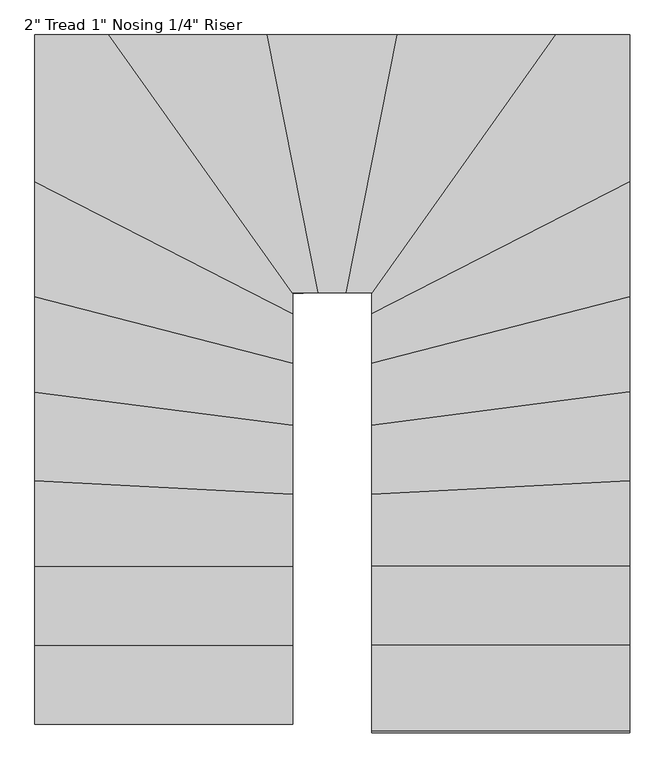
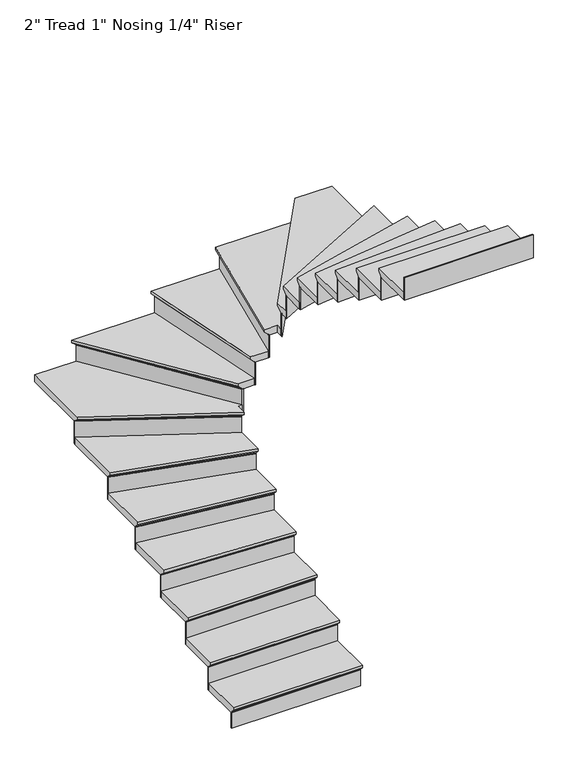
"""IFC4 building model written with IfcOpenShell, lengths in millimetres: stair flight geometry."""

from ifc_helpers import new_model, si_unit, origin, place, context, project, spatial, faceted_brep, source, transform, mapped, element, save


def stair_flight_079dc026(model_context):
    return source(origin(), model_context, "Body", "Brep", [
        faceted_brep([(-8021.860887, -4607.8089531, 150.2833333), (-8021.860887, -4607.8089531, 169.3333333), (-8936.260887, -4607.8089531, 169.3333333), (-8936.260887, -4607.8089531, 150.2833333), (-8021.860887, -4582.4089531, 124.8833333), (-8936.260887, -4582.4089531, 124.8833333), (-8021.860887, -4303.0089531, 169.3333333), (-8936.260887, -4303.0089531, 169.3333333), (-8936.260887, -4582.4089531, 118.5333333), (-8936.260887, -4303.0089531, 118.5333333), (-8021.860887, -4303.0089531, 118.5333333), (-8021.860887, -4582.4089531, 118.5333333)], [[[0, 1, 2, 3]], [[4, 0, 3, 5]], [[2, 1, 6, 7]], [[8, 9, 10, 11]], [[2, 7, 9, 8, 5, 3]], [[8, 11, 4, 5]], [[6, 1, 0, 4, 11, 10]], [[7, 6, 10, 9]]]),
        faceted_brep([(-8021.860887, -4582.4089531, 118.5333333), (-8021.860887, -4582.4089531, 0.0), (-8021.860887, -4576.0589531, 0.0), (-8021.860887, -4576.0589531, 118.5333333), (-8936.260887, -4582.4089531, 118.5333333), (-8936.260887, -4576.0589531, 118.5333333), (-8936.260887, -4576.0589531, 0.0), (-8936.260887, -4582.4089531, 0.0)], [[[0, 1, 2, 3]], [[4, 5, 6, 7]], [[1, 0, 4, 7]], [[2, 1, 7, 6]], [[3, 2, 6, 5]], [[0, 3, 5, 4]]]),
        faceted_brep([(-8021.860887, -4303.0089531, 287.8666667), (-8021.860887, -4303.0089531, 118.5333333), (-8021.860887, -4296.6589531, 118.5333333), (-8021.860887, -4296.6589531, 287.8666667), (-8936.260887, -4303.0089531, 287.8666667), (-8936.260887, -4296.6589531, 287.8666667), (-8936.260887, -4296.6589531, 118.5333333), (-8936.260887, -4303.0089531, 118.5333333)], [[[0, 1, 2, 3]], [[4, 5, 6, 7]], [[1, 0, 4, 7]], [[2, 1, 7, 6]], [[3, 2, 6, 5]], [[0, 3, 5, 4]]]),
        faceted_brep([(-8936.260887, -4328.4089531, 338.6666667), (-8021.860887, -4328.4089531, 338.6666667), (-8021.860887, -4023.6089531, 338.6666667), (-8936.260887, -4023.6089531, 338.6666667), (-8936.260887, -4303.0089531, 287.8666667), (-8936.260887, -4023.6089531, 287.8666667), (-8021.860887, -4023.6089531, 287.8666667), (-8021.860887, -4303.0089531, 287.8666667), (-8936.260887, -4303.0089531, 294.2166667), (-8936.260887, -4328.4089531, 319.6166667), (-8021.860887, -4303.0089531, 294.2166667), (-8021.860887, -4328.4089531, 319.6166667)], [[[0, 1, 2, 3]], [[4, 5, 6, 7]], [[0, 3, 5, 4, 8, 9]], [[4, 7, 10, 8]], [[2, 1, 11, 10, 7, 6]], [[3, 2, 6, 5]], [[11, 1, 0, 9]], [[10, 11, 9, 8]]]),
        faceted_brep([(-8021.860887, -4023.6089531, 457.2), (-8021.860887, -4023.6089531, 287.8666667), (-8021.860887, -4017.2589531, 287.8666667), (-8021.860887, -4017.2589531, 457.2), (-8936.260887, -4023.6089531, 457.2), (-8936.260887, -4017.2589531, 457.2), (-8936.260887, -4017.2589531, 287.8666667), (-8936.260887, -4023.6089531, 287.8666667)], [[[0, 1, 2, 3]], [[4, 5, 6, 7]], [[1, 0, 4, 7]], [[2, 1, 7, 6]], [[3, 2, 6, 5]], [[0, 3, 5, 4]]]),
        faceted_brep([(-8936.260887, -4049.0089531, 508.0), (-8021.860887, -4049.0089531, 508.0), (-8021.860887, -3767.9417916, 508.0), (-8936.260887, -3720.4075212, 508.0), (-8936.260887, -4023.6089531, 457.2), (-8936.260887, -3720.4075212, 457.2), (-8021.860887, -3767.9417916, 457.2), (-8021.860887, -4023.6089531, 457.2), (-8936.260887, -4023.6089531, 463.55), (-8936.260887, -4049.0089531, 488.95), (-8021.860887, -4023.6089531, 463.55), (-8021.860887, -4049.0089531, 488.95)], [[[0, 1, 2, 3]], [[4, 5, 6, 7]], [[0, 3, 5, 4, 8, 9]], [[4, 7, 10, 8]], [[2, 1, 11, 10, 7, 6]], [[3, 2, 6, 5]], [[11, 1, 0, 9]], [[10, 11, 9, 8]]]),
        faceted_brep([(-8021.860887, -3767.9417916, 626.5333333), (-8021.860887, -3767.9417916, 457.2), (-8021.860887, -3761.5832175, 457.2), (-8021.860887, -3761.5832175, 626.5333333), (-8936.260887, -3720.4075212, 626.5333333), (-8936.260887, -3714.0489471, 626.5333333), (-8936.260887, -3714.0489471, 457.2), (-8936.260887, -3720.4075212, 457.2)], [[[0, 1, 2, 3]], [[4, 5, 6, 7]], [[1, 0, 4, 7]], [[2, 1, 7, 6]], [[3, 2, 6, 5]], [[0, 3, 5, 4]]]),
        faceted_brep([(-8936.260887, -3745.8418179, 677.3333333), (-8021.860887, -3793.3760883, 677.3333333), (-8021.860887, -3523.7750918, 677.3333333), (-8936.260887, -3405.4190402, 677.3333333), (-8936.260887, -3720.4075212, 626.5333333), (-8936.260887, -3405.4190402, 626.5333333), (-8021.860887, -3523.7750918, 626.5333333), (-8021.860887, -3767.9417916, 626.5333333), (-8936.260887, -3720.4075212, 632.8833333), (-8936.260887, -3745.8418179, 658.2833333), (-8021.860887, -3767.9417916, 632.8833333), (-8021.860887, -3793.3760883, 658.2833333)], [[[0, 1, 2, 3]], [[4, 5, 6, 7]], [[0, 3, 5, 4, 8, 9]], [[4, 7, 10, 8]], [[2, 1, 11, 10, 7, 6]], [[3, 2, 6, 5]], [[11, 1, 0, 9]], [[10, 11, 9, 8]]]),
        faceted_brep([(-8021.860887, -3523.7750918, 795.8666667), (-8021.860887, -3523.7750918, 626.5333333), (-8021.860887, -3517.37212, 626.5333333), (-8021.860887, -3517.37212, 795.8666667), (-8936.260887, -3405.4190402, 795.8666667), (-8936.260887, -3399.0160684, 795.8666667), (-8936.260887, -3399.0160684, 626.5333333), (-8936.260887, -3405.4190402, 626.5333333)], [[[0, 1, 2, 3]], [[4, 5, 6, 7]], [[1, 0, 4, 7]], [[2, 1, 7, 6]], [[3, 2, 6, 5]], [[0, 3, 5, 4]]]),
        faceted_brep([(-8936.260887, -3431.0309273, 846.6666667), (-8021.860887, -3549.3869789, 846.6666667), (-8021.860887, -3302.1478693, 846.6666667), (-8936.260887, -3067.0174219, 846.6666667), (-8936.260887, -3405.4190402, 795.8666667), (-8936.260887, -3067.0174219, 795.8666667), (-8021.860887, -3302.1478693, 795.8666667), (-8021.860887, -3523.7750918, 795.8666667), (-8936.260887, -3405.4190402, 802.2166667), (-8936.260887, -3431.0309273, 827.6166667), (-8021.860887, -3523.7750918, 802.2166667), (-8021.860887, -3549.3869789, 827.6166667)], [[[0, 1, 2, 3]], [[4, 5, 6, 7]], [[0, 3, 5, 4, 8, 9]], [[4, 7, 10, 8]], [[2, 1, 11, 10, 7, 6]], [[3, 2, 6, 5]], [[11, 1, 0, 9]], [[10, 11, 9, 8]]]),
        faceted_brep([(-8021.860887, -3302.1478693, 965.2), (-8021.860887, -3302.1478693, 795.8666667), (-8021.860887, -3295.5912925, 795.8666667), (-8021.860887, -3295.5912925, 965.2), (-8936.260887, -3067.0174219, 965.2), (-8936.260887, -3060.4608451, 965.2), (-8936.260887, -3060.4608451, 795.8666667), (-8936.260887, -3067.0174219, 795.8666667)], [[[0, 1, 2, 3]], [[4, 5, 6, 7]], [[1, 0, 4, 7]], [[2, 1, 7, 6]], [[3, 2, 6, 5]], [[0, 3, 5, 4]]]),
        faceted_brep([(-8936.260887, -3093.2437294, 1016.0), (-8021.860887, -3328.3741768, 1016.0), (-8021.860887, -3125.8012333, 1016.0), (-8936.260887, -2656.9766119, 1016.0), (-8936.260887, -3067.0174219, 965.2), (-8936.260887, -2656.9766119, 965.2), (-8021.860887, -3125.8012333, 965.2), (-8021.860887, -3302.1478693, 965.2), (-8936.260887, -3067.0174219, 971.55), (-8936.260887, -3093.2437294, 996.95), (-8021.860887, -3302.1478693, 971.55), (-8021.860887, -3328.3741768, 996.95)], [[[0, 1, 2, 3]], [[4, 5, 6, 7]], [[0, 3, 5, 4, 8, 9]], [[4, 7, 10, 8]], [[2, 1, 11, 10, 7, 6]], [[3, 2, 6, 5]], [[11, 1, 0, 9]], [[10, 11, 9, 8]]]),
        faceted_brep([(-8021.860887, -3125.8012333, 1134.5333333), (-8021.860887, -3125.8012333, 965.2), (-8021.860887, -3118.6652501, 965.2), (-8021.860887, -3118.6652501, 1134.5333333), (-8936.260887, -2656.9766119, 1134.5333333), (-8936.260887, -2649.8406288, 1134.5333333), (-8936.260887, -2649.8406288, 965.2), (-8936.260887, -2656.9766119, 965.2)], [[[0, 1, 2, 3]], [[4, 5, 6, 7]], [[1, 0, 4, 7]], [[2, 1, 7, 6]], [[3, 2, 6, 5]], [[0, 3, 5, 4]]]),
        faceted_brep([(-8642.5797533, -2165.6772612, 1185.3333333), (-8936.260887, -2165.6772612, 1185.3333333), (-8936.260887, -2685.5205445, 1185.3333333), (-8021.860887, -3154.3451658, 1185.3333333), (-8021.860887, -3080.0772612, 1185.3333333), (-7992.3058042, -3080.0772612, 1185.3333333), (-8936.260887, -2165.6772612, 1134.5333333), (-8642.5797533, -2165.6772612, 1134.5333333), (-7992.3058042, -3080.0772612, 1134.5333333), (-8021.860887, -3080.0772612, 1134.5333333), (-8021.860887, -3125.8012333, 1134.5333333), (-8936.260887, -2656.9766119, 1134.5333333), (-8936.260887, -2656.9766119, 1140.8833333), (-8936.260887, -2685.5205445, 1166.2833333), (-8021.860887, -3125.8012333, 1140.8833333), (-8021.860887, -3154.3451658, 1166.2833333)], [[[0, 1, 2, 3, 4, 5]], [[6, 7, 8, 9, 10, 11]], [[1, 0, 7, 6]], [[2, 1, 6, 11, 12, 13]], [[11, 10, 14, 12]], [[4, 3, 15, 14, 10, 9]], [[5, 4, 9, 8]], [[0, 5, 8, 7]], [[15, 3, 2, 13]], [[14, 15, 13, 12]]]),
        faceted_brep([(-7992.3058042, -3080.0772612, 1303.8666667), (-7992.3058042, -3080.0772612, 1134.5333333), (-7984.5138294, -3080.0772612, 1134.5333333), (-7984.5138294, -3080.0772612, 1303.8666667), (-8642.5797533, -2165.6772612, 1303.8666667), (-8634.7877785, -2165.6772612, 1303.8666667), (-8634.7877785, -2165.6772612, 1134.5333333), (-8642.5797533, -2165.6772612, 1134.5333333)], [[[0, 1, 2, 3]], [[4, 5, 6, 7]], [[1, 0, 4, 7]], [[2, 1, 7, 6]], [[3, 2, 6, 5]], [[0, 3, 5, 4]]]),
        faceted_brep([(-8673.7476525, -2165.6772612, 1354.6666667), (-8023.4737034, -3080.0772612, 1354.6666667), (-7905.8517171, -3080.0772612, 1354.6666667), (-8086.0925734, -2165.6772612, 1354.6666667), (-8642.5797533, -2165.6772612, 1303.8666667), (-8086.0925734, -2165.6772612, 1303.8666667), (-7905.8517171, -3080.0772612, 1303.8666667), (-7992.3058042, -3080.0772612, 1303.8666667), (-8642.5797533, -2165.6772612, 1310.2166667), (-8673.7476525, -2165.6772612, 1335.6166667), (-7992.3058042, -3080.0772612, 1310.2166667), (-8023.4737034, -3080.0772612, 1335.6166667)], [[[0, 1, 2, 3]], [[4, 5, 6, 7]], [[0, 3, 5, 4, 8, 9]], [[4, 7, 10, 8]], [[2, 1, 11, 10, 7, 6]], [[3, 2, 6, 5]], [[11, 1, 0, 9]], [[10, 11, 9, 8]]]),
        faceted_brep([(-7905.8517171, -3080.0772612, 1473.2), (-7905.8517171, -3080.0772612, 1303.8666667), (-7899.3795317, -3080.0772612, 1303.8666667), (-7899.3795317, -3080.0772612, 1473.2), (-8086.0925734, -2165.6772612, 1473.2), (-8079.620388, -2165.6772612, 1473.2), (-8079.620388, -2165.6772612, 1303.8666667), (-8086.0925734, -2165.6772612, 1303.8666667)], [[[0, 1, 2, 3]], [[4, 5, 6, 7]], [[1, 0, 4, 7]], [[2, 1, 7, 6]], [[3, 2, 6, 5]], [[0, 3, 5, 4]]]),
        faceted_brep([(-8111.9813152, -2165.6772612, 1524.0), (-7931.7404589, -3080.0772612, 1524.0), (-7806.6925734, -3080.0772612, 1524.0), (-7626.4517171, -2165.6772612, 1524.0), (-8086.0925734, -2165.6772612, 1473.2), (-7626.4517171, -2165.6772612, 1473.2), (-7806.6925734, -3080.0772612, 1473.2), (-7905.8517171, -3080.0772612, 1473.2), (-8086.0925734, -2165.6772612, 1479.55), (-8111.9813152, -2165.6772612, 1504.95), (-7905.8517171, -3080.0772612, 1479.55), (-7931.7404589, -3080.0772612, 1504.95)], [[[0, 1, 2, 3]], [[4, 5, 6, 7]], [[0, 3, 5, 4, 8, 9]], [[4, 7, 10, 8]], [[2, 1, 11, 10, 7, 6]], [[3, 2, 6, 5]], [[11, 1, 0, 9]], [[10, 11, 9, 8]]]),
        faceted_brep([(-7806.6925734, -3080.0772612, 1642.5333333), (-7806.6925734, -3080.0772612, 1473.2), (-7800.220388, -3080.0772612, 1473.2), (-7800.220388, -3080.0772612, 1642.5333333), (-7626.4517171, -2165.6772612, 1642.5333333), (-7619.9795317, -2165.6772612, 1642.5333333), (-7619.9795317, -2165.6772612, 1473.2), (-7626.4517171, -2165.6772612, 1473.2)], [[[0, 1, 2, 3]], [[4, 5, 6, 7]], [[1, 0, 4, 7]], [[2, 1, 7, 6]], [[3, 2, 6, 5]], [[0, 3, 5, 4]]]),
        faceted_brep([(-7652.3404589, -2165.6772612, 1693.3333333), (-7832.5813152, -3080.0772612, 1693.3333333), (-7742.460887, -3080.0772612, 1693.3333333), (-7742.460887, -3126.1727358, 1693.3333333), (-7059.4062224, -2165.6772612, 1693.3333333), (-7626.4517171, -2165.6772612, 1642.5333333), (-7059.4062224, -2165.6772612, 1642.5333333), (-7742.460887, -3126.1727358, 1642.5333333), (-7742.460887, -3080.0772612, 1642.5333333), (-7806.6925734, -3080.0772612, 1642.5333333), (-7626.4517171, -2165.6772612, 1648.8833333), (-7652.3404589, -2165.6772612, 1674.2833333), (-7806.6925734, -3080.0772612, 1648.8833333), (-7832.5813152, -3080.0772612, 1674.2833333)], [[[0, 1, 2, 3, 4]], [[5, 6, 7, 8, 9]], [[0, 4, 6, 5, 10, 11]], [[5, 9, 12, 10]], [[2, 1, 13, 12, 9, 8]], [[3, 2, 8, 7]], [[4, 3, 7, 6]], [[13, 1, 0, 11]], [[12, 13, 11, 10]]]),
        faceted_brep([(-7742.460887, -3126.1727358, 1811.8666667), (-7742.460887, -3126.1727358, 1642.5333333), (-7742.460887, -3137.1296282, 1642.5333333), (-7742.460887, -3137.1296282, 1811.8666667), (-7059.4062224, -2165.6772612, 1811.8666667), (-7051.6142476, -2165.6772612, 1811.8666667), (-7051.6142476, -2165.6772612, 1642.5333333), (-7059.4062224, -2165.6772612, 1642.5333333)], [[[0, 1, 2, 3]], [[4, 5, 6, 7]], [[1, 0, 4, 7]], [[2, 1, 7, 6]], [[3, 2, 6, 5]], [[0, 3, 5, 4]]]),
        faceted_brep([(-6828.060887, -2714.064477, 1862.6666667), (-6828.060887, -2165.6772612, 1862.6666667), (-7090.5741215, -2165.6772612, 1862.6666667), (-7742.460887, -3082.3451658, 1862.6666667), (-7742.460887, -3182.8890983, 1862.6666667), (-6828.060887, -2165.6772612, 1811.8666667), (-6828.060887, -2714.064477, 1811.8666667), (-7742.460887, -3182.8890983, 1811.8666667), (-7742.460887, -3126.1727358, 1811.8666667), (-7059.4062224, -2165.6772612, 1811.8666667), (-7059.4062224, -2165.6772612, 1818.2166667), (-7090.5741215, -2165.6772612, 1843.6166667), (-7742.460887, -3126.1727358, 1818.2166667), (-7742.460887, -3082.3451658, 1843.6166667)], [[[0, 1, 2, 3, 4]], [[5, 6, 7, 8, 9]], [[1, 0, 6, 5]], [[2, 1, 5, 9, 10, 11]], [[9, 8, 12, 10]], [[4, 3, 13, 12, 8, 7]], [[0, 4, 7, 6]], [[13, 3, 2, 11]], [[12, 13, 11, 10]]]),
        faceted_brep([(-7742.460887, -3182.8890983, 1981.2), (-7742.460887, -3182.8890983, 1811.8666667), (-7742.460887, -3190.0250815, 1811.8666667), (-7742.460887, -3190.0250815, 1981.2), (-6828.060887, -2714.064477, 1981.2), (-6828.060887, -2721.2004601, 1981.2), (-6828.060887, -2721.2004601, 1811.8666667), (-6828.060887, -2714.064477, 1811.8666667)], [[[0, 1, 2, 3]], [[4, 5, 6, 7]], [[1, 0, 4, 7]], [[2, 1, 7, 6]], [[3, 2, 6, 5]], [[0, 3, 5, 4]]]),
        faceted_brep([(-6828.060887, -2685.5205445, 2032.0), (-7742.460887, -3154.3451658, 2032.0), (-7742.460887, -3354.6004843, 2032.0), (-6828.060887, -3119.4700369, 2032.0), (-6828.060887, -2714.064477, 1981.2), (-6828.060887, -3119.4700369, 1981.2), (-7742.460887, -3354.6004843, 1981.2), (-7742.460887, -3182.8890983, 1981.2), (-6828.060887, -2714.064477, 1987.55), (-6828.060887, -2685.5205445, 2012.95), (-7742.460887, -3182.8890983, 1987.55), (-7742.460887, -3154.3451658, 2012.95)], [[[0, 1, 2, 3]], [[4, 5, 6, 7]], [[0, 3, 5, 4, 8, 9]], [[4, 7, 10, 8]], [[2, 1, 11, 10, 7, 6]], [[3, 2, 6, 5]], [[11, 1, 0, 9]], [[10, 11, 9, 8]]]),
        faceted_brep([(-7742.460887, -3354.6004843, 2150.5333333), (-7742.460887, -3354.6004843, 1981.2), (-7742.460887, -3361.1570611, 1981.2), (-7742.460887, -3361.1570611, 2150.5333333), (-6828.060887, -3119.4700369, 2150.5333333), (-6828.060887, -3126.0266137, 2150.5333333), (-6828.060887, -3126.0266137, 1981.2), (-6828.060887, -3119.4700369, 1981.2)], [[[0, 1, 2, 3]], [[4, 5, 6, 7]], [[1, 0, 4, 7]], [[2, 1, 7, 6]], [[3, 2, 6, 5]], [[0, 3, 5, 4]]]),
        faceted_brep([(-6828.060887, -3093.2437294, 2201.3333333), (-7742.460887, -3328.3741768, 2201.3333333), (-7742.460887, -3574.998866, 2201.3333333), (-6828.060887, -3456.6428144, 2201.3333333), (-6828.060887, -3119.4700369, 2150.5333333), (-6828.060887, -3456.6428144, 2150.5333333), (-7742.460887, -3574.998866, 2150.5333333), (-7742.460887, -3354.6004843, 2150.5333333), (-6828.060887, -3119.4700369, 2156.8833333), (-6828.060887, -3093.2437294, 2182.2833333), (-7742.460887, -3354.6004843, 2156.8833333), (-7742.460887, -3328.3741768, 2182.2833333)], [[[0, 1, 2, 3]], [[4, 5, 6, 7]], [[0, 3, 5, 4, 8, 9]], [[4, 7, 10, 8]], [[2, 1, 11, 10, 7, 6]], [[3, 2, 6, 5]], [[11, 1, 0, 9]], [[10, 11, 9, 8]]]),
        faceted_brep([(-7742.460887, -3574.998866, 2319.8666667), (-7742.460887, -3574.998866, 2150.5333333), (-7742.460887, -3581.4018378, 2150.5333333), (-7742.460887, -3581.4018378, 2319.8666667), (-6828.060887, -3456.6428144, 2319.8666667), (-6828.060887, -3463.0457862, 2319.8666667), (-6828.060887, -3463.0457862, 2150.5333333), (-6828.060887, -3456.6428144, 2150.5333333)], [[[0, 1, 2, 3]], [[4, 5, 6, 7]], [[1, 0, 4, 7]], [[2, 1, 7, 6]], [[3, 2, 6, 5]], [[0, 3, 5, 4]]]),
        faceted_brep([(-6828.060887, -3431.0309273, 2370.6666667), (-7742.460887, -3549.3869789, 2370.6666667), (-7742.460887, -3818.810385, 2370.6666667), (-6828.060887, -3771.2761146, 2370.6666667), (-6828.060887, -3456.6428144, 2319.8666667), (-6828.060887, -3771.2761146, 2319.8666667), (-7742.460887, -3818.810385, 2319.8666667), (-7742.460887, -3574.998866, 2319.8666667), (-6828.060887, -3456.6428144, 2326.2166667), (-6828.060887, -3431.0309273, 2351.6166667), (-7742.460887, -3574.998866, 2326.2166667), (-7742.460887, -3549.3869789, 2351.6166667)], [[[0, 1, 2, 3]], [[4, 5, 6, 7]], [[0, 3, 5, 4, 8, 9]], [[4, 7, 10, 8]], [[2, 1, 11, 10, 7, 6]], [[3, 2, 6, 5]], [[11, 1, 0, 9]], [[10, 11, 9, 8]]]),
        faceted_brep([(-7742.460887, -3818.810385, 2489.2), (-7742.460887, -3818.810385, 2319.8666667), (-7742.460887, -3825.1689591, 2319.8666667), (-7742.460887, -3825.1689591, 2489.2), (-6828.060887, -3771.2761146, 2489.2), (-6828.060887, -3777.6346887, 2489.2), (-6828.060887, -3777.6346887, 2319.8666667), (-6828.060887, -3771.2761146, 2319.8666667)], [[[0, 1, 2, 3]], [[4, 5, 6, 7]], [[1, 0, 4, 7]], [[2, 1, 7, 6]], [[3, 2, 6, 5]], [[0, 3, 5, 4]]]),
        faceted_brep([(-6828.060887, -3745.8418179, 2540.0), (-7742.460887, -3793.3760883, 2540.0), (-7742.460887, -4074.4089531, 2540.0), (-6828.060887, -4074.4089531, 2540.0), (-6828.060887, -3771.2761146, 2489.2), (-6828.060887, -4074.4089531, 2489.2), (-7742.460887, -4074.4089531, 2489.2), (-7742.460887, -3818.810385, 2489.2), (-6828.060887, -3771.2761146, 2495.55), (-6828.060887, -3745.8418179, 2520.95), (-7742.460887, -3818.810385, 2495.55), (-7742.460887, -3793.3760883, 2520.95)], [[[0, 1, 2, 3]], [[4, 5, 6, 7]], [[0, 3, 5, 4, 8, 9]], [[4, 7, 10, 8]], [[2, 1, 11, 10, 7, 6]], [[3, 2, 6, 5]], [[11, 1, 0, 9]], [[10, 11, 9, 8]]]),
        faceted_brep([(-7742.460887, -4074.4089531, 2658.5333333), (-7742.460887, -4074.4089531, 2489.2), (-7742.460887, -4080.7589531, 2489.2), (-7742.460887, -4080.7589531, 2658.5333333), (-6828.060887, -4074.4089531, 2658.5333333), (-6828.060887, -4080.7589531, 2658.5333333), (-6828.060887, -4080.7589531, 2489.2), (-6828.060887, -4074.4089531, 2489.2)], [[[0, 1, 2, 3]], [[4, 5, 6, 7]], [[1, 0, 4, 7]], [[2, 1, 7, 6]], [[3, 2, 6, 5]], [[0, 3, 5, 4]]]),
        faceted_brep([(-6828.060887, -4049.0089531, 2709.3333333), (-7742.460887, -4049.0089531, 2709.3333333), (-7742.460887, -4353.8089531, 2709.3333333), (-6828.060887, -4353.8089531, 2709.3333333), (-6828.060887, -4074.4089531, 2658.5333333), (-6828.060887, -4353.8089531, 2658.5333333), (-7742.460887, -4353.8089531, 2658.5333333), (-7742.460887, -4074.4089531, 2658.5333333), (-6828.060887, -4074.4089531, 2664.8833333), (-6828.060887, -4049.0089531, 2690.2833333), (-7742.460887, -4074.4089531, 2664.8833333), (-7742.460887, -4049.0089531, 2690.2833333)], [[[0, 1, 2, 3]], [[4, 5, 6, 7]], [[0, 3, 5, 4, 8, 9]], [[4, 7, 10, 8]], [[2, 1, 11, 10, 7, 6]], [[3, 2, 6, 5]], [[11, 1, 0, 9]], [[10, 11, 9, 8]]]),
        faceted_brep([(-7742.460887, -4353.8089531, 2827.8666667), (-7742.460887, -4353.8089531, 2658.5333333), (-7742.460887, -4360.1589531, 2658.5333333), (-7742.460887, -4360.1589531, 2827.8666667), (-6828.060887, -4353.8089531, 2827.8666667), (-6828.060887, -4360.1589531, 2827.8666667), (-6828.060887, -4360.1589531, 2658.5333333), (-6828.060887, -4353.8089531, 2658.5333333)], [[[0, 1, 2, 3]], [[4, 5, 6, 7]], [[1, 0, 4, 7]], [[2, 1, 7, 6]], [[3, 2, 6, 5]], [[0, 3, 5, 4]]]),
        faceted_brep([(-7742.460887, -4633.2089531, 2997.2), (-7742.460887, -4633.2089531, 2827.8666667), (-7742.460887, -4639.5589531, 2827.8666667), (-7742.460887, -4639.5589531, 2997.2), (-6828.060887, -4633.2089531, 2997.2), (-6828.060887, -4639.5589531, 2997.2), (-6828.060887, -4639.5589531, 2827.8666667), (-6828.060887, -4633.2089531, 2827.8666667)], [[[0, 1, 2, 3]], [[4, 5, 6, 7]], [[1, 0, 4, 7]], [[2, 1, 7, 6]], [[3, 2, 6, 5]], [[0, 3, 5, 4]]]),
        faceted_brep([(-6828.060887, -4328.4089531, 2878.6666667), (-7742.460887, -4328.4089531, 2878.6666667), (-7742.460887, -4633.2089531, 2878.6666667), (-6828.060887, -4633.2089531, 2878.6666667), (-6828.060887, -4353.8089531, 2827.8666667), (-6828.060887, -4633.2089531, 2827.8666667), (-7742.460887, -4633.2089531, 2827.8666667), (-7742.460887, -4353.8089531, 2827.8666667), (-6828.060887, -4353.8089531, 2834.2166667), (-6828.060887, -4328.4089531, 2859.6166667), (-7742.460887, -4353.8089531, 2834.2166667), (-7742.460887, -4328.4089531, 2859.6166667)], [[[0, 1, 2, 3]], [[4, 5, 6, 7]], [[0, 3, 5, 4, 8, 9]], [[4, 7, 10, 8]], [[2, 1, 11, 10, 7, 6]], [[3, 2, 6, 5]], [[11, 1, 0, 9]], [[10, 11, 9, 8]]]),
    ])


if __name__ == "__main__":
    model = new_model("IFC4")
    model_context = context("Model", 3, world=origin())
    ifc_project = project(units=[si_unit("LENGTHUNIT", "METRE", prefix="MILLI")], contexts=[model_context])
    site = spatial("IfcSite", under=ifc_project)
    building = spatial("IfcBuilding", under=site)
    placement = place(None, origin())
    stair_flight_shape = stair_flight_079dc026(model_context)
    element("IfcStairFlight", 1, ObjectType="2\" Tread 1\" Nosing 1/4\" Riser", at=placement, inside=building, context=model_context, shape_type="MappedRepresentation", body=[
        mapped(stair_flight_shape, transform((0.0, 0.0, 0.0), x_axis=(1.0, 0.0, 0.0), y_axis=(0.0, 1.0, 0.0), z_axis=(0.0, 0.0, 1.0))),
    ])
    save(model, "model.ifc")
